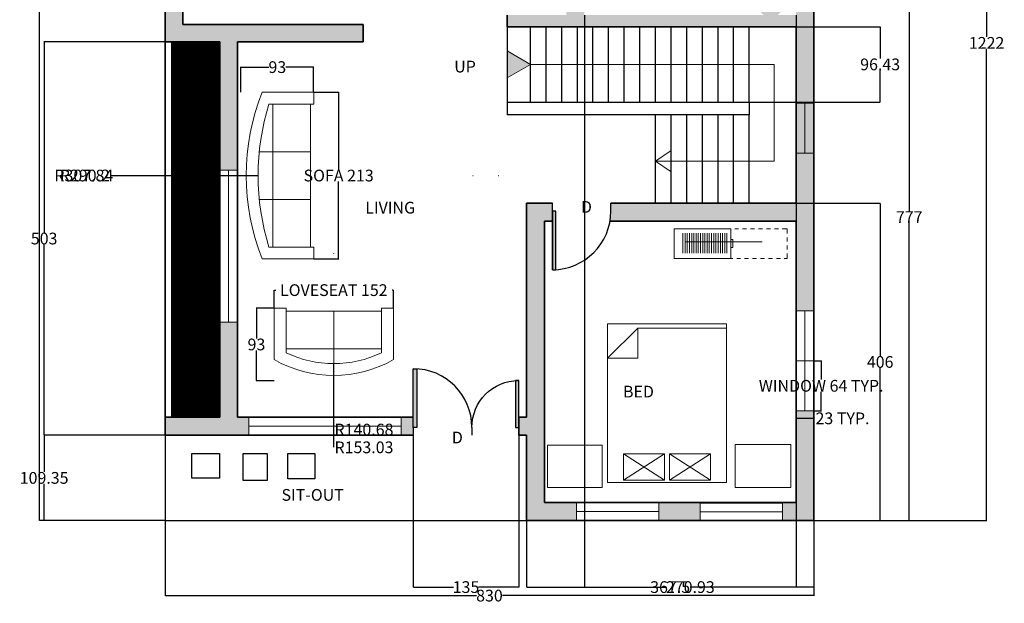
# Model space of a CAD drawing. Units: centimetres. Extents: x 355 to 1615, y 1030 to 2729.
# Tile 1 of 3: x 355 to 1615, y 1030 to 1776. Entities that reach past the tile are written whole.
import ezdxf

# ---------------------------------------------------------------- set-up
doc = ezdxf.new("R2010")
doc.units = ezdxf.units.CM
doc.header["$MEASUREMENT"] = 0
for name, color, linetype, lineweight in [('A-ANNO-DIMS', 2, 'Continuous', 18), ('A-ANNO-SYMB', 7, 'Continuous', 18), ('A-ANNO-TEXT', 7, 'Continuous', 25), ('A-AREA-IDEN', 7, 'Continuous', 25), ('A-DOOR', 4, 'Continuous', 25), ('A-FLOR', 7, 'Continuous', 25), ('A-FLOR-PATT', 252, 'Continuous', 13), ('A-FLOR-STRS', 7, 'Continuous', 25), ('A-FURN', 8, 'Continuous', 18), ('A-GLAZ', 4, 'Continuous', 18), ('A-WALL', 7, 'Continuous', 35), ('A-WALL-PATT', 5, 'Continuous', 13)]:
    doc.layers.add(name, color=color, linetype=linetype, lineweight=lineweight)
doc.styles.get("Standard").update_dxf_attribs({"font": 'arial.ttf'})
doc.dimstyles.get("Standard").update_dxf_attribs({"dimtxt": 15, "dimasz": 0.18, "dimexe": 0.18, "dimexo": 0.0625, "dimgap": 0.09, "dimtad": 0, "dimtih": 1, "dimtoh": 1, "dimdec": 0, "dimzin": 0, "dimdsep": 46, "dimtxsty": 'Standard', "dimcen": 0.09, "dimadec": 0, "dimazin": 0, "dimtfac": 1, "dimtdec": 0, "dimtofl": 0, "dimtmove": 0, "dimatfit": 3, "dimfxl": 1, "dimtolj": 1, "dimtzin": 0, "dimarcsym": 0})

# ---------------------------------------------------------------- blocks, each defined once
blk = doc.blocks.new('*U17')
for p, q in [((0, 0), (0, 100)), ((750, 0), (750, 100))]:
    blk.add_line(p, q)
blk.add_lwpolyline([(0, 0), (0, -750), (43.75, -750), (43.75, 0)], close=True)
blk.add_arc((0, 0), 750, 270, 0)
blk = doc.blocks.new('*U19')
for p, q in [((0, 0), (0, -100)), ((750, 0), (750, -100))]:
    blk.add_line(p, q)
blk.add_lwpolyline([(0, 0), (0, 750), (43.75, 750), (43.75, 0)], close=True)
blk.add_arc((0, 0), 750, 0, 90)
blk = doc.blocks.new('*U18')
for p, q in [((0, 0), (0, -100)), ((600, 0), (600, -100))]:
    blk.add_line(p, q)
blk.add_lwpolyline([(0, 0), (0, 600), (43.75, 600), (43.75, 0)], close=True)
blk.add_arc((0, 0), 600, 0, 90)
blk = doc.blocks.new('Sofa - Roundback 7 ft.')
for p, q in [((-12.00002, -32.4421), (-12.00003, -6.5971)), ((11.99997, -32.4421), (11.99998, -6.5971)), ((-36.000027, -34), (-36.000027, -11.4696)), ((-35.999844, -13.3819), (35.9998, -13.3819)), ((35.99998, -34), (35.99998, -11.4696)), ((-36.000027, -32.4421), (35.99998, -32.4421))]:
    blk.add_line(p, q)
for points in [[(-36.000027, -34), (-42.000027, -34), (-42.000027, -8)], [(41.99998, -8), (41.99998, -34), (35.99998, -34)]]:
    blk.add_lwpolyline(points)
for centre, radius, start, end in [((0, -114.25), 114.25, 68.43141, 111.5686), ((-0.00001, -127.1968), 121.1968, 72.72033, 107.2797)]:
    blk.add_arc(centre, radius, start, end)
blk = doc.blocks.new('Sofa - Roundback Loveseat 5 ft.')
for p, q in [((0, -32.44198), (0, -5.99998)), ((-24, -33.99998), (-24, -11.46958)), ((-23.9998, -13.38178), (23.99986, -13.38178)), ((24.00004, -33.99998), (24.00004, -11.46958)), ((-24, -32.44198), (24.00004, -32.44198))]:
    blk.add_line(p, q)
for points in [[(-24, -33.99998), (-30, -33.99998), (-30, -7.99998)], [(30.00004, -7.99998), (30.00004, -33.99998), (24.00004, -33.99998)]]:
    blk.add_lwpolyline(points)
for centre, radius, start, end in [((0, -60.24998), 60.24998, 60.13715, 119.8628), ((0, -61.38438), 55.38444, 64.32083, 115.6792)]:
    blk.add_arc(centre, radius, start, end)
blk = doc.blocks.new('*D28')
at = {"layer": 'A-ANNO-DIMS', "color": 0, "lineweight": -2, "transparency": 16777216}
for p, q in [((1371.3, 1912.2), (1493.7, 1912.2)), ((1493.5, 1912), (1493.5, 1531.3)), ((1493.5, 1135.5), (1493.5, 1516.2)), ((1371.3, 1135.3), (1493.7, 1135.3))]:
    blk.add_line(p, q, dxfattribs=at)
at = {"layer": 'A-ANNO-DIMS', "color": 0, "transparency": 16777216}
for points in [[(1493.5, 1912), (1493.5, 1912), (1493.5, 1912.2)], [(1493.5, 1135.5), (1493.5, 1135.5), (1493.5, 1135.3)]]:
    blk.add_solid(points, dxfattribs=at)
at = {"layer": 'Defpoints', "color": 0, "transparency": 16777216}
for p in [(1371.2, 1912.2), (1371.2, 1135.3), (1493.5, 1135.3)]:
    blk.add_point(p, dxfattribs=at)
at = {"layer": 'A-ANNO-DIMS', "color": 0, "transparency": 16777216, "insert": (1493.5, 1523.7), "char_height": 15, "attachment_point": 5}
blk.add_mtext('\\A1;777', dxfattribs=at)
blk = doc.blocks.new('*D29')
at = {"layer": 'A-ANNO-DIMS', "color": 0, "lineweight": -2, "transparency": 16777216}
for p, q in [((1371.3, 2357.7), (1592.7, 2357.7)), ((1592.5, 2357.5), (1592.5, 1754.1)), ((1592.5, 1135.5), (1592.5, 1738.9)), ((1371.3, 1135.3), (1592.7, 1135.3))]:
    blk.add_line(p, q, dxfattribs=at)
at = {"layer": 'A-ANNO-DIMS', "color": 0, "transparency": 16777216}
for points in [[(1592.4, 2357.5), (1592.5, 2357.5), (1592.5, 2357.7)], [(1592.4, 1135.5), (1592.5, 1135.5), (1592.5, 1135.3)]]:
    blk.add_solid(points, dxfattribs=at)
at = {"layer": 'Defpoints', "color": 0, "transparency": 16777216}
for p in [(1371.2, 2357.7), (1371.2, 1135.3), (1592.5, 1135.3)]:
    blk.add_point(p, dxfattribs=at)
at = {"layer": 'A-ANNO-DIMS', "color": 0, "transparency": 16777216, "insert": (1592.5, 1746.5), "char_height": 15, "attachment_point": 5}
blk.add_mtext('\\A1;1222', dxfattribs=at)
blk = doc.blocks.new('*D30')
at = {"layer": 'A-ANNO-DIMS', "color": 0, "lineweight": -2, "transparency": 16777216}
for p, q in [((541.2, 1135.3), (541.2, 1039.2)), ((1371.2, 1135.3), (1371.2, 1039.2)), ((541.4, 1039.4), (939.6, 1039.4)), ((1371.1, 1039.4), (972.9, 1039.4))]:
    blk.add_line(p, q, dxfattribs=at)
at = {"layer": 'A-ANNO-DIMS', "color": 0, "transparency": 16777216}
for points in [[(541.4, 1039.4), (541.4, 1039.4), (541.2, 1039.4)], [(1371.1, 1039.4), (1371.1, 1039.4), (1371.2, 1039.4)]]:
    blk.add_solid(points, dxfattribs=at)
at = {"layer": 'Defpoints', "color": 0, "transparency": 16777216}
for p in [(541.2, 1135.3), (1371.2, 1135.3), (1371.2, 1039.4)]:
    blk.add_point(p, dxfattribs=at)
at = {"layer": 'A-ANNO-DIMS', "color": 0, "transparency": 16777216, "insert": (956.2, 1039.4), "char_height": 15, "attachment_point": 5}
blk.add_mtext('\\A1;830', dxfattribs=at)
blk = doc.blocks.new('*D31')
at = {"layer": 'A-ANNO-DIMS', "color": 0, "lineweight": -2, "transparency": 16777216}
for p, q in [((611.2, 2537.7), (380.2, 2537.7)), ((380.4, 2537.5), (380.4, 1844.2)), ((380.4, 1135.5), (380.4, 1828.7)), ((541.2, 1135.3), (380.2, 1135.3))]:
    blk.add_line(p, q, dxfattribs=at)
at = {"layer": 'A-ANNO-DIMS', "color": 0, "transparency": 16777216}
for points in [[(380.4, 2537.5), (380.4, 2537.5), (380.4, 2537.7)], [(380.4, 1135.5), (380.4, 1135.5), (380.4, 1135.3)]]:
    blk.add_solid(points, dxfattribs=at)
at = {"layer": 'Defpoints', "color": 0, "transparency": 16777216}
for p in [(380.4, 2537.7), (611.2, 2537.7), (541.2, 1135.3)]:
    blk.add_point(p, dxfattribs=at)
at = {"layer": 'A-ANNO-DIMS', "color": 0, "transparency": 16777216, "insert": (380.4, 1836.5), "char_height": 15, "attachment_point": 5}
blk.add_mtext('\\A1;1402', dxfattribs=at)
blk = doc.blocks.new('BED-QUEEN-WITH-NIGHTSTANDS')
for p, q in [((82.2, 0), (82.2, 203.2)), ((82.2, 203.2), (234.6, 203.2)), ((234.6, 203.2), (234.6, 0)), ((102.6, 200.2), (155.4, 200.2)), ((102.6, 166.6), (102.6, 200.2)), ((102.6, 200.2), (155.4, 166.6)), ((102.6, 166.6), (155.4, 200.2)), ((155.4, 200.2), (155.4, 166.6)), ((161.5, 200.2), (214.3, 200.2)), ((161.5, 166.6), (161.5, 200.2)), ((161.5, 200.2), (214.3, 166.6)), ((161.5, 166.6), (214.3, 200.2)), ((214.3, 200.2), (214.3, 166.6)), ((155.4, 166.6), (102.6, 166.6)), ((161.5, 166.6), (214.3, 166.6)), ((234.6, 44.3), (196, 5.7)), ((196, 44.3), (234.6, 44.3)), ((196, 5.7), (196, 44.3)), ((82.2, 5.7), (196, 5.7)), ((234.6, 0), (82.2, 0))]:
    blk.add_line(p, q)
for points in [[(71.2, 209.5), (0, 209.5), (0, 154.4), (71.2, 154.4)], [(241.3, 209.5), (311.6, 209.5), (311.6, 155.3), (241.3, 155.3)]]:
    blk.add_lwpolyline(points, close=True)
blk = doc.blocks.new('File Cabinet - Letter')
for p, q in [((0, 0), (15, 0)), ((0, -28.5), (0, 0)), ((15, 0), (15, -28.5)), ((15, -28.5), (0, -28.5)), ((0, -29.5), (0, -28.5)), ((5.5, -28.5), (5.5, -29.5)), ((5.5, -29.5), (9.5, -29.5)), ((9.5, -29.5), (9.5, -28.5)), ((0, -33.5), (0, -31.5)), ((15, -30.5), (15, -32.5)), ((15, -34.5), (15, -36.5)), ((0, -37.5), (0, -35.5)), ((0, -41.5), (0, -39.5)), ((15, -38.5), (15, -40.5)), ((0, -45.5), (0, -43.5)), ((15, -42.5), (15, -44.5)), ((0, -49.5), (0, -47.5)), ((15, -46.5), (15, -48.5)), ((0, -53.5), (0, -51.5)), ((15, -50.5), (15, -52.5)), ((15, -54.5), (15, -57)), ((0, -57), (0, -55.5)), ((2.5, -57), (0, -57)), ((6.5, -57), (4.5, -57)), ((10.5, -57), (8.5, -57)), ((15, -57), (12.5, -57))]:
    blk.add_line(p, q)
blk = doc.blocks.new('BEDROOM-STORAGE-CABINET')
for p, q in [((11.1, 32.6), (11.1, 6.7)), ((13.9, 32.6), (13.9, 6.7)), ((16.7, 32.6), (16.7, 6.7)), ((19.6, 32.6), (19.6, 6.7)), ((22.4, 32.6), (22.4, 6.7)), ((25.2, 32.6), (25.2, 6.7)), ((28, 32.6), (28, 6.7)), ((30.9, 32.6), (30.9, 6.7)), ((33.7, 32.6), (33.7, 6.7)), ((36.5, 32.6), (36.5, 6.7)), ((39.3, 32.6), (39.3, 6.7)), ((42.2, 32.6), (42.2, 6.7)), ((45, 32.6), (45, 6.7)), ((47.8, 32.6), (47.8, 6.7)), ((50.6, 32.6), (50.6, 6.7)), ((53.5, 32.6), (53.5, 6.7)), ((56.3, 32.6), (56.3, 6.7)), ((59.1, 32.6), (59.1, 6.7)), ((61.9, 32.6), (61.9, 6.7)), ((64.8, 32.6), (64.8, 6.7)), ((67.6, 32.6), (67.6, 6.7)), ((13.9, 21.3), (112.8, 21.3))]:
    blk.add_line(p, q)
at = {"xscale": 2.54, "yscale": 2.54, "zscale": 2.54, "rotation": 90}
blk.add_blockref('File Cabinet - Letter', (0, 0), dxfattribs=at)
blk = doc.blocks.new('WIN-1949')
blk.add_line((194.8, 11.2), (0, 11.2))
blk.add_lwpolyline([(0, 22.5), (194.8, 22.5), (194.8, 0), (0, 0)], close=True)
blk = doc.blocks.new('WIN-1054')
blk.add_line((0, 11.2), (105.4, 11.2))
blk.add_lwpolyline([(0, 22.5), (105.4, 22.5), (105.4, 0), (0, 0)], close=True)
blk = doc.blocks.new('WIN-640')
blk.add_line((11.3, 64), (11.3, 0))
blk.add_lwpolyline([(0, 64), (22.5, 64), (22.5, 0), (0, 0)], close=True)
blk = doc.blocks.new('*D40')
at = {"layer": 'A-ANNO-DIMS', "color": 0, "lineweight": -2, "transparency": 16777216}
for p, q in [((1371.3, 1339.8), (1381, 1339.8)), ((1380.8, 1339.6), (1380.8, 1315.7)), ((1380.8, 1276), (1380.8, 1299.9)), ((1371.3, 1275.8), (1381, 1275.8))]:
    blk.add_line(p, q, dxfattribs=at)
at = {"layer": 'A-ANNO-DIMS', "color": 0, "transparency": 16777216}
for points in [[(1380.8, 1339.6), (1380.9, 1339.6), (1380.8, 1339.8)], [(1380.8, 1276), (1380.9, 1276), (1380.8, 1275.8)]]:
    blk.add_solid(points, dxfattribs=at)
at = {"layer": 'Defpoints', "color": 0, "transparency": 16777216}
for p in [(1371.2, 1339.8), (1380.8, 1339.8), (1371.2, 1275.8)]:
    blk.add_point(p, dxfattribs=at)
at = {"layer": 'A-ANNO-DIMS', "color": 0, "transparency": 16777216, "insert": (1380.8, 1307.8), "char_height": 15, "attachment_point": 5}
blk.add_mtext('\\A1;WINDOW 64 TYP.', dxfattribs=at)
blk = doc.blocks.new('*D41')
at = {"layer": 'A-ANNO-DIMS', "color": 0, "lineweight": -2, "transparency": 16777216}
for p, q in [((1348.7, 1275.7), (1348.7, 1266)), ((1371.2, 1275.7), (1371.2, 1266)), ((1348.9, 1266.2), (1371.1, 1266.2)), ((1371.2, 1266.2), (1371.4, 1266.2))]:
    blk.add_line(p, q, dxfattribs=at)
at = {"layer": 'A-ANNO-DIMS', "color": 0, "transparency": 16777216}
for points in [[(1348.9, 1266.2), (1348.9, 1266.1), (1348.7, 1266.2)], [(1371.1, 1266.2), (1371.1, 1266.1), (1371.2, 1266.2)]]:
    blk.add_solid(points, dxfattribs=at)
at = {"layer": 'Defpoints', "color": 0, "transparency": 16777216}
for p in [(1348.7, 1275.8), (1371.2, 1275.8), (1371.2, 1266.2)]:
    blk.add_point(p, dxfattribs=at)
at = {"layer": 'A-ANNO-DIMS', "color": 0, "transparency": 16777216, "insert": (1408.1, 1266.2), "char_height": 15, "attachment_point": 5}
blk.add_mtext('\\A1;23 TYP.', dxfattribs=at)
blk = doc.blocks.new('*D60')
at = {"layer": 'A-ANNO-DIMS', "color": 0, "lineweight": -2, "transparency": 16777216}
for p, q in [((731.3, 1683.5), (763.4, 1683.5)), ((763.2, 1683.3), (763.2, 1584.7)), ((763.2, 1470.3), (763.2, 1569)), ((731.3, 1470.1), (763.4, 1470.1))]:
    blk.add_line(p, q, dxfattribs=at)
at = {"layer": 'A-ANNO-DIMS', "color": 0, "transparency": 16777216}
for points in [[(763.2, 1683.3), (763.3, 1683.3), (763.2, 1683.5)], [(763.2, 1470.3), (763.3, 1470.3), (763.2, 1470.1)]]:
    blk.add_solid(points, dxfattribs=at)
at = {"layer": 'Defpoints', "color": 0, "transparency": 16777216}
for p in [(731.2, 1683.5), (763.2, 1683.5), (731.2, 1470.1)]:
    blk.add_point(p, dxfattribs=at)
at = {"layer": 'A-ANNO-DIMS', "color": 0, "transparency": 16777216, "insert": (763.2, 1576.8), "char_height": 15, "attachment_point": 5}
blk.add_mtext('\\A1;SOFA 213', dxfattribs=at)
blk = doc.blocks.new('*D61')
at = {"layer": 'A-ANNO-DIMS', "color": 0, "lineweight": -2, "transparency": 16777216}
for p, q in [((638.1, 1683.6), (638.1, 1715.7)), ((638.3, 1715.5), (673.8, 1715.5)), ((731, 1715.5), (695.5, 1715.5)), ((731.2, 1683.6), (731.2, 1715.7))]:
    blk.add_line(p, q, dxfattribs=at)
at = {"layer": 'A-ANNO-DIMS', "color": 0, "transparency": 16777216}
for points in [[(638.3, 1715.5), (638.3, 1715.5), (638.1, 1715.5)], [(731, 1715.5), (731, 1715.5), (731.2, 1715.5)]]:
    blk.add_solid(points, dxfattribs=at)
at = {"layer": 'Defpoints', "color": 0, "transparency": 16777216}
for p in [(638.1, 1715.5), (638.1, 1683.5), (731.2, 1683.5)]:
    blk.add_point(p, dxfattribs=at)
at = {"layer": 'A-ANNO-DIMS', "color": 0, "transparency": 16777216, "insert": (684.7, 1715.5), "char_height": 15, "attachment_point": 5}
blk.add_mtext('\\A1;93', dxfattribs=at)
blk = doc.blocks.new('*D62')
at = {"layer": 'A-ANNO-DIMS', "color": 0, "lineweight": -2, "transparency": 16777216}
for p, q in [((680.8, 1407.4), (680.8, 1430.3)), ((681, 1430.2), (682.6, 1430.2)), ((833.1, 1430.2), (831.5, 1430.2)), ((833.2, 1407.4), (833.2, 1430.3))]:
    blk.add_line(p, q, dxfattribs=at)
at = {"layer": 'A-ANNO-DIMS', "color": 0, "transparency": 16777216}
for points in [[(681, 1430.2), (681, 1430.1), (680.8, 1430.2)], [(833.1, 1430.2), (833.1, 1430.1), (833.2, 1430.2)]]:
    blk.add_solid(points, dxfattribs=at)
at = {"layer": 'Defpoints', "color": 0, "transparency": 16777216}
for p in [(680.8, 1430.2), (680.8, 1407.3), (833.2, 1407.3)]:
    blk.add_point(p, dxfattribs=at)
at = {"layer": 'A-ANNO-DIMS', "color": 0, "transparency": 16777216, "insert": (757, 1430.2), "char_height": 15, "attachment_point": 5}
blk.add_mtext('\\A1;LOVESEAT 152', dxfattribs=at)
blk = doc.blocks.new('*D63')
at = {"layer": 'A-ANNO-DIMS', "color": 0, "lineweight": -2, "transparency": 16777216}
for p, q in [((680.8, 1407.3), (657.8, 1407.3)), ((658, 1407.1), (658, 1368.5)), ((658, 1314.4), (658, 1353)), ((680.8, 1314.2), (657.8, 1314.2))]:
    blk.add_line(p, q, dxfattribs=at)
at = {"layer": 'A-ANNO-DIMS', "color": 0, "transparency": 16777216}
for points in [[(657.9, 1407.1), (658, 1407.1), (658, 1407.3)], [(657.9, 1314.4), (658, 1314.4), (658, 1314.2)]]:
    blk.add_solid(points, dxfattribs=at)
at = {"layer": 'Defpoints', "color": 0, "transparency": 16777216}
for p in [(680.8, 1407.3), (658, 1314.2), (680.8, 1314.2)]:
    blk.add_point(p, dxfattribs=at)
at = {"layer": 'A-ANNO-DIMS', "color": 0, "transparency": 16777216, "insert": (658, 1360.7), "char_height": 15, "attachment_point": 5}
blk.add_mtext('\\A1;93', dxfattribs=at)
blk = doc.blocks.new('*D65')
at = {"layer": 'A-ANNO-DIMS', "color": 0, "lineweight": -2, "transparency": 16777216}
for p, q in [((1348.8, 1541.3), (1456.5, 1541.3)), ((1456.3, 1541.1), (1456.3, 1346.1)), ((1456.3, 1135.5), (1456.3, 1330.6)), ((1371.3, 1135.3), (1456.5, 1135.3))]:
    blk.add_line(p, q, dxfattribs=at)
at = {"layer": 'A-ANNO-DIMS', "color": 0, "transparency": 16777216}
for points in [[(1456.3, 1541.1), (1456.3, 1541.1), (1456.3, 1541.3)], [(1456.3, 1135.5), (1456.3, 1135.5), (1456.3, 1135.3)]]:
    blk.add_solid(points, dxfattribs=at)
at = {"layer": 'Defpoints', "color": 0, "transparency": 16777216}
for p in [(1348.7, 1541.3), (1456.3, 1541.3), (1371.2, 1135.3)]:
    blk.add_point(p, dxfattribs=at)
at = {"layer": 'A-ANNO-DIMS', "color": 0, "transparency": 16777216, "insert": (1456.3, 1338.3), "char_height": 15, "attachment_point": 5}
blk.add_mtext('\\A1;406', dxfattribs=at)
blk = doc.blocks.new('*D66')
at = {"layer": 'A-ANNO-DIMS', "color": 0, "lineweight": -2, "transparency": 16777216}
for p, q in [((1077.8, 1782.1), (1077.8, 1050.1)), ((1348.7, 1782.1), (1348.7, 1050.1)), ((1078, 1050.3), (1181.9, 1050.3)), ((1348.6, 1050.3), (1244.6, 1050.3))]:
    blk.add_line(p, q, dxfattribs=at)
at = {"layer": 'A-ANNO-DIMS', "color": 0, "transparency": 16777216}
for points in [[(1078, 1050.3), (1078, 1050.2), (1077.8, 1050.3)], [(1348.6, 1050.3), (1348.6, 1050.2), (1348.7, 1050.3)]]:
    blk.add_solid(points, dxfattribs=at)
at = {"layer": 'Defpoints', "color": 0, "transparency": 16777216}
for p in [(1077.8, 1782.2), (1348.7, 1782.2), (1348.7, 1050.3)]:
    blk.add_point(p, dxfattribs=at)
at = {"layer": 'A-ANNO-DIMS', "color": 0, "transparency": 16777216, "insert": (1213.3, 1050.3), "char_height": 15, "attachment_point": 5}
blk.add_mtext('\\A1;270.93', dxfattribs=at)
blk = doc.blocks.new('*D68')
at = {"layer": 'A-ANNO-DIMS', "color": 0, "lineweight": -2, "transparency": 16777216}
for p, q in [((541.2, 1244.7), (386, 1244.7)), ((386.2, 1244.5), (386.2, 1197.8)), ((386.2, 1135.5), (386.2, 1182.2)), ((541.2, 1135.3), (386, 1135.3))]:
    blk.add_line(p, q, dxfattribs=at)
at = {"layer": 'A-ANNO-DIMS', "color": 0, "transparency": 16777216}
for points in [[(386.2, 1244.5), (386.2, 1244.5), (386.2, 1244.7)], [(386.2, 1135.5), (386.2, 1135.5), (386.2, 1135.3)]]:
    blk.add_solid(points, dxfattribs=at)
at = {"layer": 'Defpoints', "color": 0, "transparency": 16777216}
for p in [(386.2, 1244.7), (541.2, 1244.7), (541.2, 1135.3)]:
    blk.add_point(p, dxfattribs=at)
at = {"layer": 'A-ANNO-DIMS', "color": 0, "transparency": 16777216, "insert": (386.2, 1190), "char_height": 15, "attachment_point": 5}
blk.add_mtext('\\A1;109.35', dxfattribs=at)
blk = doc.blocks.new('*D69')
at = {"layer": 'A-ANNO-DIMS', "color": 0, "lineweight": -2, "transparency": 16777216}
for p, q in [((858.7, 1244.6), (858.7, 1050.1)), ((993.7, 1244.6), (993.7, 1050.1)), ((858.9, 1050.3), (910.2, 1050.3)), ((993.6, 1050.3), (942.2, 1050.3))]:
    blk.add_line(p, q, dxfattribs=at)
at = {"layer": 'A-ANNO-DIMS', "color": 0, "transparency": 16777216}
for points in [[(858.9, 1050.3), (858.9, 1050.2), (858.7, 1050.3)], [(993.6, 1050.3), (993.6, 1050.2), (993.7, 1050.3)]]:
    blk.add_solid(points, dxfattribs=at)
at = {"layer": 'Defpoints', "color": 0, "transparency": 16777216}
for p in [(858.7, 1244.7), (993.7, 1244.7), (993.7, 1050.3)]:
    blk.add_point(p, dxfattribs=at)
at = {"layer": 'A-ANNO-DIMS', "color": 0, "transparency": 16777216, "insert": (926.2, 1050.3), "char_height": 15, "attachment_point": 5}
blk.add_mtext('\\A1;135', dxfattribs=at)
blk = doc.blocks.new('*D71')
at = {"layer": 'A-ANNO-DIMS', "color": 0, "lineweight": -2, "transparency": 16777216}
for p, q in [((1288.8, 1767.2), (1456.5, 1767.2)), ((1456.3, 1767), (1456.3, 1726.7)), ((1456.3, 1670.9), (1456.3, 1711.2)), ((1288.8, 1670.7), (1456.5, 1670.7))]:
    blk.add_line(p, q, dxfattribs=at)
at = {"layer": 'A-ANNO-DIMS', "color": 0, "transparency": 16777216}
for points in [[(1456.3, 1767), (1456.3, 1767), (1456.3, 1767.2)], [(1456.3, 1670.9), (1456.3, 1670.9), (1456.3, 1670.7)]]:
    blk.add_solid(points, dxfattribs=at)
at = {"layer": 'Defpoints', "color": 0, "transparency": 16777216}
for p in [(1288.7, 1767.2), (1456.3, 1767.2), (1288.7, 1670.7)]:
    blk.add_point(p, dxfattribs=at)
at = {"layer": 'A-ANNO-DIMS', "color": 0, "transparency": 16777216, "insert": (1456.3, 1719), "char_height": 15, "attachment_point": 5}
blk.add_mtext('\\A1;96.43', dxfattribs=at)
blk = doc.blocks.new('*D73')
at = {"layer": 'A-ANNO-DIMS', "color": 0, "lineweight": -2, "transparency": 16777216}
for p, q in [((1003.7, 1135.3), (1003.7, 1050.1)), ((1371.2, 1135.3), (1371.2, 1050.1)), ((1003.9, 1050.3), (1162, 1050.3)), ((1371.1, 1050.3), (1212.9, 1050.3))]:
    blk.add_line(p, q, dxfattribs=at)
at = {"layer": 'A-ANNO-DIMS', "color": 0, "transparency": 16777216}
for points in [[(1003.9, 1050.3), (1003.9, 1050.2), (1003.7, 1050.3)], [(1371.1, 1050.3), (1371.1, 1050.2), (1371.2, 1050.3)]]:
    blk.add_solid(points, dxfattribs=at)
at = {"layer": 'Defpoints', "color": 0, "transparency": 16777216}
for p in [(1003.7, 1135.3), (1371.2, 1135.3), (1371.2, 1050.3)]:
    blk.add_point(p, dxfattribs=at)
at = {"layer": 'A-ANNO-DIMS', "color": 0, "transparency": 16777216, "insert": (1187.5, 1050.3), "char_height": 15, "attachment_point": 5}
blk.add_mtext('\\A1;367.5', dxfattribs=at)
blk = doc.blocks.new('*D74')
at = {"layer": 'A-ANNO-DIMS', "color": 0, "lineweight": -2, "transparency": 16777216}
for p, q in [((541.2, 1747.7), (386, 1747.7)), ((386.2, 1747.5), (386.2, 1503.9)), ((386.2, 1244.9), (386.2, 1488.4)), ((541.2, 1244.7), (386, 1244.7))]:
    blk.add_line(p, q, dxfattribs=at)
at = {"layer": 'A-ANNO-DIMS', "color": 0, "transparency": 16777216}
for points in [[(386.2, 1747.5), (386.2, 1747.5), (386.2, 1747.7)], [(386.2, 1244.9), (386.2, 1244.9), (386.2, 1244.7)]]:
    blk.add_solid(points, dxfattribs=at)
at = {"layer": 'Defpoints', "color": 0, "transparency": 16777216}
for p in [(541.2, 1747.7), (386.2, 1244.7), (541.2, 1244.7)]:
    blk.add_point(p, dxfattribs=at)
at = {"layer": 'A-ANNO-DIMS', "color": 0, "transparency": 16777216, "insert": (386.2, 1496.2), "char_height": 15, "attachment_point": 5}
blk.add_mtext('\\A1;503', dxfattribs=at)
blk = doc.blocks.new('*D76')
at = {"layer": 'A-ANNO-DIMS', "color": 0, "lineweight": -2, "transparency": 16777216}
for p, q in [((475.4, 1576.8), (659.9, 1576.8)), ((967.9, 1576.7), (967.9, 1576.9)), ((967.9, 1576.8), (968, 1576.8))]:
    blk.add_line(p, q, dxfattribs=at)
at = {"layer": 'A-ANNO-DIMS', "color": 0, "transparency": 16777216}
blk.add_solid([(659.9, 1576.8), (659.9, 1576.8), (660.1, 1576.8)], dxfattribs=at)
at = {"layer": 'Defpoints', "color": 0, "transparency": 16777216}
for p in [(660.1, 1576.8), (967.9, 1576.8)]:
    blk.add_point(p, dxfattribs=at)
at = {"layer": 'A-ANNO-DIMS', "color": 0, "transparency": 16777216, "insert": (437, 1576.8), "char_height": 15, "attachment_point": 5}
blk.add_mtext('\\A1;R307.84', dxfattribs=at)
blk = doc.blocks.new('*D77')
at = {"layer": 'A-ANNO-DIMS', "color": 0, "lineweight": -2, "transparency": 16777216}
for p, q in [((470.7, 1576.8), (644.7, 1576.8)), ((935, 1576.8), (935.2, 1576.8)), ((935.1, 1576.7), (935.1, 1576.9))]:
    blk.add_line(p, q, dxfattribs=at)
at = {"layer": 'A-ANNO-DIMS', "color": 0, "transparency": 16777216}
blk.add_solid([(644.7, 1576.8), (644.7, 1576.8), (644.9, 1576.8)], dxfattribs=at)
at = {"layer": 'Defpoints', "color": 0, "transparency": 16777216}
for p in [(644.9, 1576.8), (935.1, 1576.8)]:
    blk.add_point(p, dxfattribs=at)
at = {"layer": 'A-ANNO-DIMS', "color": 0, "transparency": 16777216, "insert": (438.3, 1576.8), "char_height": 15, "attachment_point": 5}
blk.add_mtext('\\A1;R290.2', dxfattribs=at)
blk = doc.blocks.new('*D78')
at = {"layer": 'A-ANNO-DIMS', "color": 0, "lineweight": -2, "transparency": 16777216}
for p, q in [((756.9, 1474), (757.1, 1474)), ((757, 1473.9), (757, 1474.1)), ((757, 1229.1), (757, 1320.8)), ((757.2, 1229.1), (757, 1229.1))]:
    blk.add_line(p, q, dxfattribs=at)
at = {"layer": 'A-ANNO-DIMS', "color": 0, "transparency": 16777216}
blk.add_solid([(757.1, 1320.8), (757, 1320.8), (757, 1320.9)], dxfattribs=at)
at = {"layer": 'Defpoints', "color": 0, "transparency": 16777216}
for p in [(757, 1474), (757, 1320.9)]:
    blk.add_point(p, dxfattribs=at)
at = {"layer": 'A-ANNO-DIMS', "color": 0, "transparency": 16777216, "insert": (795.6, 1229.1), "char_height": 15, "attachment_point": 5}
blk.add_mtext('\\A1;R153.03', dxfattribs=at)
blk = doc.blocks.new('*D79')
at = {"layer": 'A-ANNO-DIMS', "color": 0, "lineweight": -2, "transparency": 16777216}
for p, q in [((756.9, 1476.9), (757.1, 1476.9)), ((757, 1476.8), (757, 1477)), ((757, 1251.8), (757, 1336)), ((757.2, 1251.8), (757, 1251.8))]:
    blk.add_line(p, q, dxfattribs=at)
at = {"layer": 'A-ANNO-DIMS', "color": 0, "transparency": 16777216}
blk.add_solid([(757.1, 1336), (757, 1336), (757, 1336.2)], dxfattribs=at)
at = {"layer": 'Defpoints', "color": 0, "transparency": 16777216}
for p in [(757, 1476.9), (757, 1336.2)]:
    blk.add_point(p, dxfattribs=at)
at = {"layer": 'A-ANNO-DIMS', "color": 0, "transparency": 16777216, "insert": (795.6, 1251.8), "char_height": 15, "attachment_point": 5}
blk.add_mtext('\\A1;R140.68', dxfattribs=at)

msp = doc.modelspace()

# ---------------------------------------------------------------- hatches: boundary and pattern name
at = {"layer": 'A-ANNO-SYMB'}
h = msp.add_hatch(color=256, dxfattribs=at)
h.dxf.hatch_style = 1
h.paths.add_polyline_path([(978.7322, 1736.2768), (978.7322, 1701.6358), (1008.7322, 1718.9563)])
at = {"layer": 'A-FLOR-PATT'}
h = msp.add_hatch(dxfattribs=at)
h.set_pattern_fill('ANSI32', color=256)
h.paths.add_polyline_path([(611.2322, 1747.6708), (549.2322, 1747.6708), (549.2322, 1267.6708), (611.2322, 1267.6708), (611.2322, 1388.9888), (611.1948, 1388.9888), (611.1948, 1583.8272)])
h = msp.add_hatch(color=256, dxfattribs=at)
h.set_gradient(color1=(0, 0, 255), color2=(255, 255, 0), centered=1, tint=1)
h.paths.add_polyline_path([(549.2322, 1267.6708), (611.2322, 1267.6708), (611.2322, 1388.9888), (611.1948, 1388.9888), (611.1948, 1583.8272), (611.2322, 1747.6708), (549.2322, 1747.6708)])
at = {"layer": 'A-WALL-PATT'}
h = msp.add_hatch(color=256, dxfattribs=at)
h.dxf.hatch_style = 1
h.paths.add_polyline_path([(611.2322, 1747.6708), (611.2322, 1583.8272), (633.7322, 1583.8272), (633.7322, 1747.6708), (794.4619, 1747.6708), (794.4619, 1770.1708), (563.7322, 1770.1708), (563.7322, 1828.1708), (471.2322, 1828.1708), (471.2322, 1805.1708), (541.2322, 1805.1708), (541.2322, 1747.6708)])
h.paths.add_polyline_path([(1371.2322, 2048.5797), (1348.7322, 2048.5797), (1348.7322, 1935.1708), (1147.8044, 1935.1708), (1147.8044, 1925.1708, -0.054654003), (1146.3791, 1912.1708), (1348.7322, 1912.1708), (1348.7322, 1889.2147), (1371.2322, 1889.2147)])
h.paths.add_polyline_path([(988.2322, 1945.1708), (988.2322, 1949.5458), (1078.2322, 1949.5458), (1078.2322, 1945.1708), (1001.2322, 1945.1708), (1001.2322, 1935.1708), (1087.8044, 1935.1708), (1087.8044, 1925.1708), (1092.1794, 1925.1708), (1092.1794, 1865.1708), (1087.8044, 1865.1708), (1087.8044, 1912.1708), (1077.8044, 1912.1708), (1077.8044, 1782.1708), (1306.9174, 1782.1708), (1302.395, 1786.6932), (1302.395, 1823.4958), (1288.6113, 1837.2795, -0.079615576), (1310.6652, 1842.5806), (1310.6652, 1840.9346), (1321.6922, 1840.9346), (1321.6922, 1841.147), (1321.6922, 1842.5806, -0.079615576), (1343.7462, 1837.2795), (1329.9624, 1823.4958), (1329.9624, 1786.6932), (1325.44, 1782.1708), (1348.7322, 1782.1708), (1348.7322, 1889.2147), (1371.2322, 1889.2147), (1371.2322, 1605.3038), (1348.7322, 1605.3038), (1348.7322, 1767.1708), (978.7322, 1767.1708), (978.7322, 1782.1708), (1054.8044, 1782.1708), (1054.8044, 1912.1708), (978.2322, 1912.1708), (978.2322, 1945.1708)])
h.paths.add_polyline_path([(1371.2322, 1605.3038), (1348.7322, 1605.3038), (1348.7322, 1541.3252), (1111.7322, 1541.3252), (1111.7322, 1531.3252, -0.043580868), (1110.5969, 1518.3252), (1348.7322, 1518.3252), (1348.7322, 1403.9189), (1371.2322, 1403.9189)])
h.paths.add_polyline_path([(1173.1703, 1158.3252), (1173.1703, 1135.3252), (1225.9516, 1135.3252), (1225.9516, 1158.3252)])
h.paths.add_polyline_path([(648.3142, 1244.6708), (648.3142, 1267.6708), (633.7322, 1267.6708), (633.7322, 1388.9888), (611.2322, 1388.9888), (611.2322, 1267.6708), (541.2322, 1267.6708), (541.2322, 1244.6708)])
h.paths.add_polyline_path([(633.7322, 2117.6708), (633.7322, 2127.6708), (621.2322, 2127.6708), (611.2322, 2127.6708), (611.2322, 2117.6708), (541.2322, 2117.6708), (541.2322, 2060.1708), (471.2322, 2060.1708), (471.2322, 2037.1708), (563.7322, 2037.1708), (563.7322, 2095.1708), (878.7322, 2095.1708), (878.7322, 2105.1708, -0.034848932), (879.6045, 2117.6708)])
h.paths.add_polyline_path([(843.1527, 1267.3404), (843.1527, 1244.8404), (648.3142, 1244.8404), (648.3142, 1244.6708), (858.7322, 1244.6708), (858.7322, 1254.6708), (863.1072, 1254.6708), (863.1072, 1329.6708), (858.7322, 1329.6708), (858.7322, 1267.6708), (648.3142, 1267.6708), (648.3142, 1267.3404)])
h.paths.add_polyline_path([(1067.7288, 1135.8252), (1067.7288, 1158.3252), (1026.7322, 1158.3252), (1026.7322, 1518.3252), (1036.7322, 1518.3252), (1036.7322, 1456.3252), (1041.1072, 1456.3252), (1041.1072, 1531.3252), (1036.7322, 1531.3252), (1036.7322, 1541.3252), (1003.7322, 1541.3252), (1003.7322, 1267.6708), (993.7322, 1267.6708), (993.7322, 1314.6708), (989.3572, 1314.6708), (989.3572, 1254.6708), (993.7322, 1254.6708), (993.7322, 1244.6708), (1003.7322, 1244.6708), (1003.7322, 1135.3252), (1173.1703, 1135.3252), (1173.1703, 1135.8252)])
msp.add_hatch(color=256, dxfattribs=at).paths.add_polyline_path([(1371.2322, 1275.7757), (1348.7322, 1275.7757), (1348.7322, 1158.3252), (1331.3931, 1158.3252), (1331.3931, 1135.3252), (1371.2322, 1135.3252)])

# ---------------------------------------------------------------- linework, layer by layer
at = {"layer": 'A-ANNO-SYMB'}
for p, q in [((1008.7322, 1718.9563), (1320.5534, 1718.9563)), ((1320.5534, 1718.9563), (1320.5534, 1595.1034)), ((1168.7322, 1595.1034), (1188.7322, 1608.8106)), ((1320.5534, 1595.1034), (1168.7322, 1595.1034)), ((1168.7322, 1595.1034), (1188.7322, 1581.3963))]:
    msp.add_line(p, q, dxfattribs=at)
msp.add_lwpolyline([(1008.7322, 1718.9563), (978.7322, 1736.2768), (978.7322, 1701.6358)], close=True, dxfattribs=at)
at = {"layer": 'A-DOOR'}
msp.add_line((1036.7322, 1456.3252), (1036.7322, 1541.3252), dxfattribs=at)
at = {"layer": 'A-FLOR'}
msp.add_line((549.2322, 1747.6708), (549.2322, 1267.6708), dxfattribs=at)
msp.add_lwpolyline([(541.2322, 1244.6708), (541.2322, 1135.3252), (1003.7322, 1135.3252)], dxfattribs=at)
for points in [[(575.1672, 1221.0398), (610.5806, 1221.0398), (610.5806, 1189.5981), (575.1672, 1189.5981)], [(641.0755, 1221.0398), (671.5704, 1221.0398), (671.5704, 1186.6504), (641.0755, 1186.6504)], [(698.1305, 1221.0398), (732.5602, 1221.0398), (732.5602, 1188.6155), (698.1305, 1188.6155)]]:
    msp.add_lwpolyline(points, close=True, dxfattribs=at)
at = {"layer": 'A-FLOR-STRS'}
for p, q in [((978.7322, 1767.1708), (978.7322, 1654.248)), ((1008.7322, 1670.7418), (1008.7322, 1767.1708)), ((1028.7322, 1670.7418), (1028.7322, 1767.1708)), ((1048.7322, 1670.7418), (1048.7322, 1767.1708)), ((1068.7322, 1670.7418), (1068.7322, 1767.1708)), ((1088.7322, 1670.7418), (1088.7322, 1767.1708)), ((1108.7322, 1670.7418), (1108.7322, 1767.1708)), ((1128.7322, 1670.7418), (1128.7322, 1767.1708)), ((1148.7322, 1670.7418), (1148.7322, 1767.1708)), ((1168.7322, 1670.7418), (1168.7322, 1767.1708)), ((1188.7322, 1670.7418), (1188.7322, 1767.1708)), ((1208.7322, 1670.7418), (1208.7322, 1767.1708)), ((1228.7322, 1670.7418), (1228.7322, 1767.1708)), ((1248.7322, 1670.7418), (1248.7322, 1767.1708)), ((1268.7322, 1670.7418), (1268.7322, 1767.1708)), ((1288.7322, 1670.7418), (1288.7322, 1767.1708)), ((1288.7322, 1670.7418), (1288.7322, 1654.248)), ((1168.7322, 1541.3252), (1168.7322, 1654.248)), ((1188.7322, 1541.3252), (1188.7322, 1654.248)), ((1208.7322, 1541.3252), (1208.7322, 1654.248)), ((1228.7322, 1541.3252), (1228.7322, 1654.248)), ((1248.7322, 1541.3252), (1248.7322, 1654.248)), ((1268.7322, 1541.3252), (1268.7322, 1654.248)), ((1288.7322, 1541.3252), (1288.7322, 1654.248))]:
    msp.add_line(p, q, dxfattribs=at)
for points in [[(978.7322, 1670.7418), (1288.7322, 1670.7418)], [(1288.7322, 1654.248), (978.7322, 1654.248)]]:
    msp.add_lwpolyline(points, dxfattribs=at)
at = {"layer": 'A-WALL'}
for p, q in [((1371.2322, 1135.3252), (1371.2322, 2357.6708)), ((563.7322, 2095.1708), (563.7322, 1770.1708)), ((541.2322, 1805.1708), (541.2322, 1244.6708)), ((978.7322, 1782.1708), (978.7322, 1767.1708)), ((563.7322, 1770.1708), (794.4619, 1770.1708)), ((794.4619, 1770.1708), (794.4619, 1747.6708)), ((978.7322, 1767.1708), (1348.7322, 1767.1708)), ((1348.7322, 1541.3252), (1348.7322, 1767.1708)), ((541.2322, 1747.6708), (611.2322, 1747.6708)), ((611.2322, 1747.6708), (611.2322, 1267.6708)), ((633.7322, 1747.6708), (633.7322, 1267.6708)), ((633.7322, 1747.6708), (794.4619, 1747.6708)), ((633.7322, 1267.6708), (633.7322, 1747.6708)), ((633.7322, 1747.6708), (794.4619, 1747.6708)), ((1003.7322, 1541.3252), (1003.7322, 1267.6708)), ((1003.7322, 1541.3252), (1036.7322, 1541.3252)), ((1111.7322, 1541.3252), (1348.7322, 1541.3252)), ((1026.7322, 1518.3252), (1026.7322, 1244.6708)), ((1026.7322, 1158.3252), (1026.7322, 1518.3252)), ((1026.7322, 1518.3252), (1036.7322, 1518.3252)), ((1110.5969, 1518.3252), (1348.7322, 1518.3252)), ((1348.7322, 1158.3252), (1348.7322, 1518.3252)), ((611.2322, 1267.6708), (541.2322, 1267.6708)), ((858.7322, 1267.6708), (633.7322, 1267.6708)), ((1003.7322, 1267.6708), (993.7322, 1267.6708)), ((993.7322, 1267.6708), (993.7322, 1244.6708)), ((858.7322, 1244.6708), (541.2322, 1244.6708)), ((1003.7322, 1244.6708), (993.7322, 1244.6708)), ((1348.7322, 1158.3252), (1026.7322, 1158.3252))]:
    msp.add_line(p, q, dxfattribs=at)
for points in [[(1003.7322, 1267.6708), (1003.7322, 1541.3252)], [(1371.2322, 1135.3252), (1003.7322, 1135.3252), (1003.7322, 1244.6708)]]:
    msp.add_lwpolyline(points, dxfattribs=at)

# ---------------------------------------------------------------- block references
at = {"layer": 'A-DOOR', "yscale": 0.1, "zscale": 0.1}
for name, p, xscale in [('*U17', (1036.7322, 1531.3252), 0.1), ('*U19', (858.7322, 1254.6708), 0.1), ('*U18', (993.7322, 1254.6708), -0.1)]:
    msp.add_blockref(name, p, dxfattribs=dict(at, xscale=xscale))
at = {"layer": 'A-FURN', "xscale": 2.54, "yscale": 2.54, "zscale": 2.54}
for name, p, rotation in [('Sofa - Roundback 7 ft.', (644.8669, 1576.8087), 90), ('Sofa - Roundback Loveseat 5 ft.', (757.0327, 1320.9495), 180)]:
    msp.add_blockref(name, p, dxfattribs=dict(at, rotation=rotation))
at = {"layer": 'A-FURN'}
msp.add_blockref('BEDROOM-STORAGE-CABINET', (1192.628, 1470.6848), dxfattribs=at)
at = {"layer": 'A-FURN', "rotation": 180}
msp.add_blockref('BED-QUEEN-WITH-NIGHTSTANDS', (1341.9273, 1387.2803), dxfattribs=at)
at = {"layer": 'A-GLAZ'}
for name, p in [('WIN-640', (1348.732, 1605.3039)), ('WIN-640', (1348.732, 1339.8712)), ('WIN-640', (1348.732, 1275.7759)), ('WIN-1949', (648.3138, 1244.8406)), ('WIN-1054', (1067.7291, 1135.8254)), ('WIN-1054', (1225.9519, 1135.3254))]:
    msp.add_blockref(name, p, dxfattribs=at)
at = {"layer": 'A-GLAZ', "rotation": 269.9999999999999}
msp.add_blockref('WIN-1949', (611.195, 1583.8276), dxfattribs=at)

# ---------------------------------------------------------------- texts
at = {"layer": 'A-ANNO-TEXT', "char_height": 15, "attachment_point": 1}
for s, width, insert in [('UP', 89.241844, (911.0945, 1723.6651)), ('D', 33.654124, (1073.3131, 1544.1552)), ('D', 33.654124, (908.1092, 1249.1528))]:
    msp.add_mtext_dynamic_manual_height_columns(s, width=width, gutter_width=1, heights=[0], dxfattribs=dict(at, insert=insert))
at = {"layer": 'A-AREA-IDEN', "char_height": 15, "attachment_point": 1}
for s, insert in [('LIVING ', (797.2281, 1543.1982)), ('BED', (1127.1496, 1307.8909)), ('SIT-OUT', (690.0626, 1175.7502))]:
    msp.add_mtext_dynamic_manual_height_columns(s, width=89.241844, gutter_width=1, heights=[0], dxfattribs=dict(at, insert=insert))

# ---------------------------------------------------------------- dimensions: what is measured, and where the dimension line sits
at = {"layer": 'A-ANNO-DIMS'}
for base, p1, p2, angle, override, picture, middle in [((380.4137, 2537.6708), (541.2322, 1135.3252), (611.2322, 2537.6708), 90, {"dimclrd": 0, "dimclre": 0, "dimclrt": 0}, '*D31', (380.4137, 1836.498)), ((1592.4723, 1135.3252), (1371.2322, 2357.6708), (1371.2322, 1135.3252), 90, {"dimclrd": 0, "dimclre": 0, "dimclrt": 0}, '*D29', (1592.4723, 1746.498)), ((1493.5127, 1135.3252), (1371.2322, 1912.1708), (1371.2322, 1135.3252), 90, {"dimclrd": 0, "dimclre": 0, "dimclrt": 0}, '*D28', (1493.5127, 1523.748)), ((1456.2822, 1767.1708), (1288.7322, 1670.7418), (1288.7322, 1767.1708), 90, {"dimdec": 2, "dimlfac": 1, "dimrnd": 0, "dimzin": 0, "dimdsep": 46, "dimlunit": 2}, '*D71', (1456.2822, 1718.9563)), ((386.1822, 1244.6708), (541.2322, 1747.6708), (541.2322, 1244.6708), 90, {"dimdec": 0, "dimlfac": 1, "dimrnd": 0, "dimzin": 0, "dimdsep": 46, "dimlunit": 2}, '*D74', (386.1822, 1496.1708)), ((638.0936, 1715.4927), (731.2269, 1683.4887), (638.0936, 1683.4887), 180, {"dimdec": 0, "dimlfac": 1, "dimrnd": 0, "dimzin": 0, "dimdsep": 46, "dimlunit": 2}, '*D61', (684.6602, 1715.4927)), ((1456.2822, 1541.3252), (1371.2322, 1135.3252), (1348.7322, 1541.3252), 90, {"dimdec": 0, "dimlfac": 1, "dimrnd": 0, "dimzin": 0, "dimdsep": 46, "dimlunit": 2}, '*D65', (1456.2822, 1338.3252)), ((657.9726, 1314.1761), (680.8326, 1407.3094), (680.8326, 1314.1761), 270, {"dimdec": 0, "dimlfac": 1, "dimrnd": 0, "dimzin": 0, "dimdsep": 46, "dimlunit": 2}, '*D63', (657.9726, 1360.7428)), ((386.1822, 1244.6708), (541.2322, 1135.3252), (541.2322, 1244.6708), 90, {"dimdec": 2, "dimlfac": 1, "dimrnd": 0, "dimzin": 0, "dimdsep": 46, "dimlunit": 2}, '*D68', (386.1822, 1189.998))]:
    dim = msp.add_linear_dim(base=base, p1=p1, p2=p2, angle=angle, dimstyle='Standard', override=override, dxfattribs=at)
    dim.commit()
    dim.dimension.update_dxf_attribs({"geometry": picture, "text_midpoint": middle})
for base, p1, p2, override, picture, middle in [((1348.7322, 1050.2752), (1077.8044, 1782.1708), (1348.7322, 1782.1708), {"dimdec": 2, "dimlfac": 1, "dimrnd": 0, "dimzin": 0, "dimdsep": 46, "dimlunit": 2}, '*D66', (1213.2683, 1050.2752)), ((993.7322, 1050.2752), (858.7322, 1244.6708), (993.7322, 1244.6708), {"dimdec": 0, "dimlfac": 1, "dimrnd": 0, "dimzin": 0, "dimdsep": 46, "dimlunit": 2}, '*D69', (926.2322, 1050.2752)), ((1371.2322, 1039.4067), (541.2322, 1135.3252), (1371.2322, 1135.3252), {"dimclrd": 0, "dimclre": 0, "dimclrt": 0}, '*D30', (956.2322, 1039.4067)), ((1371.2322, 1050.2752), (1003.7322, 1135.3252), (1371.2322, 1135.3252), {"dimdec": 1, "dimlfac": 1, "dimrnd": 0, "dimzin": 0, "dimdsep": 46, "dimlunit": 2}, '*D73', (1187.4822, 1050.2752))]:
    dim = msp.add_linear_dim(base=base, p1=p1, p2=p2, dimstyle='Standard', override=override, dxfattribs=at)
    dim.commit()
    dim.dimension.update_dxf_attribs({"geometry": picture, "text_midpoint": middle})
for base, p1, p2, angle, text, picture, middle in [((763.2309, 1683.4887), (731.2269, 1470.1286), (731.2269, 1683.4887), 90, 'SOFA <>', '*D60', (763.2309, 1576.8087)), ((680.8326, 1430.1694), (833.2327, 1407.3094), (680.8326, 1407.3094), 180, 'LOVESEAT <>', '*D62', (757.0327, 1430.1694)), ((1380.8394, 1339.8236), (1371.2322, 1275.7757), (1371.2322, 1339.8236), 90, 'WINDOW <> TYP.', '*D40', (1380.8394, 1307.7996))]:
    dim = msp.add_linear_dim(base=base, p1=p1, p2=p2, angle=angle, text=text, dimstyle='Standard', override={"dimdec": 0, "dimlfac": 1, "dimrnd": 0, "dimzin": 0, "dimdsep": 46, "dimlunit": 2}, dxfattribs=at)
    dim.commit()
    dim.dimension.update_dxf_attribs({"geometry": picture, "text_midpoint": middle})
for center, mpoint, override, picture, middle in [((967.9468, 1576.8087), (660.1069, 1576.809), {"dimdec": 2, "dimlfac": 1, "dimrnd": 0, "dimzin": 0, "dimdsep": 46, "dimlunit": 2}, '*D76', (475.403, 1576.8092)), ((935.0619, 1576.8087), (644.8669, 1576.809), {"dimdec": 1, "dimlfac": 1, "dimrnd": 0, "dimzin": 0, "dimdsep": 46, "dimlunit": 2}, '*D77', (470.7499, 1576.8092)), ((757.0327, 1476.8658), (757.033, 1336.1893), {"dimdec": 2, "dimlfac": 1, "dimrnd": 0, "dimzin": 0, "dimdsep": 46, "dimlunit": 2}, '*D79', (795.6319, 1251.7834)), ((757.0327, 1473.9844), (757.033, 1320.9495), {"dimdec": 2, "dimlfac": 1, "dimrnd": 0, "dimzin": 0, "dimdsep": 46, "dimlunit": 2}, '*D78', (795.6166, 1229.1285))]:
    dim = msp.add_radius_dim(center=center, mpoint=mpoint, dimstyle='Standard', override=override, dxfattribs=at)
    dim.commit()
    dim.dimension.update_dxf_attribs({"geometry": picture, "text_midpoint": middle, "dimtype": 164})
dim = msp.add_linear_dim(base=(1371.2322031806, 1266.1685360902), p1=(1348.7322031806, 1275.7757127914), p2=(1371.2322031806, 1275.7757127914), text='<> TYP.', dimstyle='Standard', override={"dimdec": 0, "dimlfac": 1, "dimrnd": 0, "dimzin": 0, "dimdsep": 46, "dimlunit": 2}, dxfattribs=at)
dim.commit()
dim.dimension.update_dxf_attribs({"geometry": '*D41', "text_midpoint": (1408.1376056363, 1266.1685360902)})

doc.saveas('drawing.dxf')
